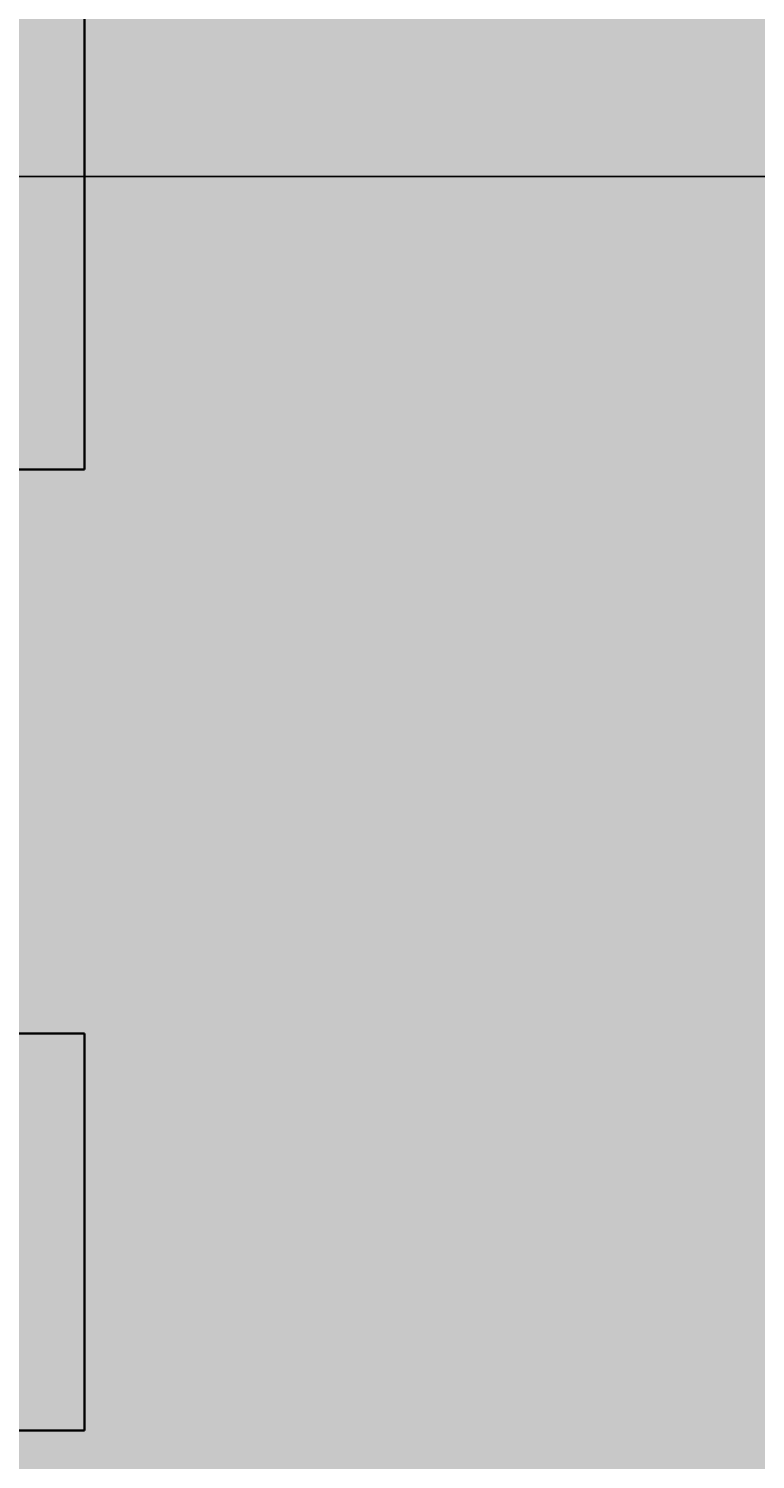
# Model space of a CAD drawing. Units: millimetres. Extents: x -229 to 16545, y -10488 to 4272.
# Tile 10 of 29: x 5862 to 7347, y -1268 to 1656. Entities that reach past the tile are written whole.
import ezdxf

# ---------------------------------------------------------------- set-up
doc = ezdxf.new("R2010")
doc.units = ezdxf.units.MM
doc.layers.add('A-ANNO-DIMS', color=2, linetype='Continuous', lineweight=18)
doc.layers.add('A-WALL', color=7, linetype='Continuous', lineweight=35)
doc.layers.add('A-FLOR-PATT', color=254, linetype='Continuous', lineweight=13, true_color=0xfeeab9)
doc.layers.add('A-WALL-PATT', color=18, linetype='Continuous', lineweight=13, true_color=0x000000)
doc.styles.get("Standard").update_dxf_attribs({"font": 'arial.ttf'})
doc.dimstyles.get("Standard").update_dxf_attribs({"dimtxt": 0.18, "dimasz": 0.18, "dimexe": 0.18, "dimexo": 0.0625, "dimgap": 0.09, "dimtad": 0, "dimtih": 1, "dimtoh": 1, "dimdec": 4, "dimzin": 0, "dimdsep": 46, "dimtxsty": 'Standard', "dimcen": 0.09, "dimadec": 0, "dimazin": 0, "dimtfac": 1, "dimtdec": 4, "dimtofl": 0, "dimtmove": 0, "dimatfit": 3, "dimfxl": 1, "dimtolj": 1, "dimtzin": 0, "dimarcsym": 0})

# ---------------------------------------------------------------- blocks, each defined once
blk = doc.blocks.new('*D85')
at = {"layer": 'A-ANNO-DIMS', "color": 0, "lineweight": -2, "transparency": 16777216}
for p, q in [((5745.9, 755.6), (5745.9, 4271.7)), ((5746.1, 4271.5), (5860.6, 4271.5)), ((5975.8, 4271.5), (5861.2, 4271.5)), ((5975.9, 755.6), (5975.9, 4271.7))]:
    blk.add_line(p, q, dxfattribs=at)
at = {"layer": 'A-ANNO-DIMS', "color": 0, "transparency": 16777216}
for points in [[(5746.1, 4271.5), (5746.1, 4271.4), (5745.9, 4271.5)], [(5975.8, 4271.5), (5975.8, 4271.4), (5975.9, 4271.5)]]:
    blk.add_solid(points, dxfattribs=at)
at = {"layer": 'Defpoints', "color": 0, "transparency": 16777216}
for p in [(5975.9, 4271.5), (5745.9, 755.5), (5975.9, 755.5)]:
    blk.add_point(p, dxfattribs=at)
at = {"layer": 'A-ANNO-DIMS', "color": 0, "transparency": 16777216, "insert": (5860.9, 4271.5), "char_height": 0.18, "attachment_point": 5}
blk.add_mtext('\\A1;230', dxfattribs=at)
blk = doc.blocks.new('*D100')
at = {"layer": 'A-ANNO-DIMS', "color": 0, "lineweight": -2, "transparency": 16777216}
for p, q in [((7294.4, 2021.7), (-228.8, 2021.7)), ((-228.7, 2021.5), (-228.7, 1688.2)), ((-228.7, 1354.6), (-228.7, 1687.9)), ((8024.8, 1354.4), (-228.8, 1354.4))]:
    blk.add_line(p, q, dxfattribs=at)
at = {"layer": 'A-ANNO-DIMS', "color": 0, "transparency": 16777216}
for points in [[(-228.7, 2021.5), (-228.6, 2021.5), (-228.7, 2021.7)], [(-228.7, 1354.6), (-228.6, 1354.6), (-228.7, 1354.4)]]:
    blk.add_solid(points, dxfattribs=at)
at = {"layer": 'Defpoints', "color": 0, "transparency": 16777216}
for p in [(7294.4, 2021.7), (-228.7, 1354.4), (8024.9, 1354.4)]:
    blk.add_point(p, dxfattribs=at)
at = {"layer": 'A-ANNO-DIMS', "color": 0, "transparency": 16777216, "insert": (-228.7, 1688.1), "char_height": 0.18, "attachment_point": 5}
blk.add_mtext('\\A1;667.3', dxfattribs=at)

msp = doc.modelspace()

# ---------------------------------------------------------------- hatches: boundary and pattern name
at = {"layer": 'A-FLOR-PATT', "transparency": 33554592}
h = msp.add_hatch(color=256, dxfattribs=at)
h.dxf.hatch_style = 1
h.paths.add_polyline_path([(7975.933, -5325.772), (7943.121, -5325.772), (7943.121, -4576.49, 0.40145271), (7225.933, -5325.772, 0.40145271), (6508.746, -4576.49), (6508.746, -5325.772), (6475.933, -5325.772), (6475.933, -5438.272), (5975.933, -5438.272), (5975.933, -7267.724), (5975.933, -7438.272), (6478.619, -7438.272), (6463.448, -7355.919), (6464.88, -7356.837), (6463.849, -7358.097), (6478.619, -7438.272), (6610.327, -7438.272), (6632.656, -7409.564), (6632.525, -7406.967), (6634.208, -7407.569), (6619.273, -7426.77), (6654.466, -7438.272), (7610.517, -7438.272), (7607.41, -7421.409), (7608.842, -7422.327), (7607.812, -7423.587), (7610.517, -7438.272), (7975.933, -7438.272)])
h.paths.add_polyline_path([(13785.933, -1208.272), (9555.933, -1208.272), (9555.933, -961.785), (9705.933, -961.785), (9705.933, -918.035), (10704.976, -918.035, 0.40145271), (9705.933, 38.215), (9555.933, 38.215), (9555.933, 2021.728), (5975.933, 2021.728), (5975.933, 755.492), (5745.933, 755.492), (5745.933, 1427.266), (2918.813, 1427.266), (2918.813, -492.942), (5013.319, -492.942), (5013.319, -978.272), (5745.933, -978.272), (5745.933, -397.513), (5975.933, -397.513), (5975.933, -1208.272), (4560.933, -1208.272), (4560.933, -1265.772), (4448.433, -1265.772), (4448.433, -1298.585), (4445.933, -1298.585), (3699.151, -1298.585, 0.40145271), (4448.433, -2015.772), (4560.933, -2015.772), (4560.933, -2384.177), (5745.933, -2384.177), (5799.402, -2384.177), (5799.402, -4518.272), (5975.933, -4518.272), (5975.933, -5208.272), (6475.933, -5208.272), (6475.933, -4575.772), (6508.746, -4575.772), (6508.746, -4576.49, -0.35647263), (7216.672, -5208.272), (7235.194, -5208.272, -0.35647263), (7943.121, -4576.49), (7943.121, -4575.772), (7975.933, -4575.772), (7975.933, -5208.272), (11176.247, -5208.272), (11159.44, -5191.465), (10520.768, -5191.465), (10520.768, -4888.936), (10571.19, -4888.936), (10571.19, -4872.129), (10772.876, -4872.129), (10772.876, -4888.936), (10789.683, -4888.936), (10789.683, -4872.129), (10991.368, -4872.129), (10991.368, -4888.936), (11041.79, -4888.936), (11041.79, -4872.129), (11058.597, -4872.129, -0.09090909), (11428.354, -4872.129), (11445.162, -4872.129), (11445.162, -4888.936), (11529.197, -4888.936), (11529.197, -5191.465), (11327.512, -5191.465), (11310.704, -5208.272), (13785.933, -5208.272)])
h.paths.add_polyline_path([(11047.216, -1630.944, -1), (11402.816, -1630.944, -1)], flags=16)
h.paths.add_polyline_path([(11148.816, -1630.944), (11225.016, -1554.744), (11301.216, -1630.944), (11225.016, -1707.144)], flags=0)
h.paths.add_polyline_path([(11199.616, -1630.944, -1), (11250.416, -1630.944, -1)], flags=0)
h.paths.add_polyline_path([(11588.751, -2096.259), (11588.751, -1543.254, -0.26666697), (12864.918, -1543.254), (12864.918, -2096.259), (12737.302, -2096.259), (12737.302, -2063.121), (11716.368, -2063.121), (11716.368, -2096.259)], flags=16)
h.paths.add_polyline_path([(12012.696, -2489.42), (12600.997, -2489.42), (12600.997, -3666.022), (12012.696, -3666.022)], flags=16)
h.paths.add_polyline_path([(12176.41, -3599.403), (12174.938, -3609.076), (12173.789, -3618.819), (12173.09, -3628.559), (12172.973, -3638.221), (12173.89, -3652.852), (12175.008, -3657.025), (12172.909, -3643.473), (12173.142, -3624.297), (12175.386, -3605.273)], flags=0)
h.paths.add_polyline_path([(8026.289, -286.944), (7737.703, -287.19), (7734.87, -269.156), (8029.092, -268.905)], flags=16)
h.paths.add_polyline_path([(7733.453, -260.139), (7710.784, -115.865), (7557.191, -115.996), (7556.999, 109.744), (7412.687, 132.166), (7412.433, 429.206), (7556.707, 451.876), (7556.568, 614.769), (7412.256, 637.19), (7412.003, 934.231), (7556.276, 956.9), (7556.084, 1182.639), (7709.677, 1182.77), (7732.099, 1327.082), (8029.14, 1327.335), (8051.808, 1183.062), (8205.401, 1183.192), (8205.594, 957.454), (8349.906, 935.031), (8350.159, 637.99), (8205.885, 615.322), (8206.024, 452.43), (8350.336, 430.006), (8350.59, 132.965), (8206.316, 110.298), (8206.509, -115.442), (8052.916, -115.573), (8030.493, -259.885)], flags=16)
h.paths.add_polyline_path([(12261.416, -3475.554), (12262.632, -3486.776), (12264.032, -3497.007), (12265.554, -3506.365), (12267.136, -3514.968), (12268.719, -3522.935), (12271.304, -3535.59), (12273.606, -3548.078), (12275.271, -3561.064), (12275.93, -3574.938), (12275.325, -3590.3), (12273.425, -3607.964), (12270.795, -3625.658), (12268.066, -3641.063), (12266.318, -3649.679), (12265.456, -3653.626), (12263.984, -3659.846), (12264.032, -3659.566), (12264.342, -3658.241), (12264.807, -3656.37), (12265.456, -3653.626), (12266.318, -3649.679), (12267.409, -3644.302), (12268.668, -3637.664), (12270.019, -3630.037), (12271.384, -3621.695), (12272.69, -3612.908), (12273.857, -3603.948), (12274.81, -3595.088), (12275.47, -3586.601), (12275.782, -3578.689), (12275.757, -3571.292), (12275.423, -3564.275), (12274.816, -3557.512), (12273.964, -3550.872), (12272.896, -3544.224), (12271.645, -3537.439), (12270.24, -3530.385), (12267.543, -3517.181), (12264.612, -3501.247), (12261.849, -3481.059)], flags=0)
h.paths.add_polyline_path([(12332.136, -3408.03), (12333.483, -3416.79), (12335.077, -3424.54), (12336.915, -3431.355), (12338.991, -3437.32), (12341.266, -3442.55), (12343.694, -3447.166), (12346.229, -3451.292), (12348.826, -3455.051), (12351.438, -3458.563), (12357.476, -3466.491), (12363.61, -3476.575), (12368.309, -3489.762), (12369.929, -3503.427), (12369.842, -3516.511), (12368.43, -3530.867), (12365.816, -3545.835), (12362.382, -3559.786), (12360.968, -3564.487), (12363.063, -3557.021), (12364.898, -3549.566), (12366.473, -3542.077), (12367.773, -3534.631), (12368.781, -3527.301), (12369.483, -3520.162), (12369.863, -3513.291), (12369.906, -3506.759), (12369.599, -3500.643), (12368.93, -3494.999), (12367.924, -3489.796), (12366.61, -3484.994), (12365.024, -3480.542), (12363.19, -3476.399), (12361.141, -3472.516), (12358.909, -3468.847), (12356.525, -3465.347), (12354.02, -3461.954), (12351.438, -3458.563), (12345.462, -3450.529), (12339.923, -3439.996), (12335.85, -3428.296), (12332.68, -3412.888)], flags=0)
h.paths.add_polyline_path([(12385.287, -3334.612), (12384.977, -3342.409), (12385.02, -3349.196), (12385.4, -3355.066), (12386.104, -3360.105), (12387.112, -3364.41), (12388.412, -3368.071), (12389.987, -3371.181), (12391.823, -3373.832), (12393.919, -3376.097), (12396.337, -3377.978), (12399.153, -3379.462), (12402.445, -3380.531), (12406.289, -3381.172), (12410.758, -3381.371), (12415.935, -3381.106), (12421.893, -3380.368), (12428.658, -3379.159), (12436.069, -3377.55), (12443.907, -3375.635), (12451.961, -3373.505), (12460.015, -3371.254), (12467.853, -3368.971), (12475.263, -3366.749), (12482.029, -3364.68), (12491.877, -3361.657), (12497.701, -3360.107), (12501.639, -3359.288), (12510.135, -3358.326), (12519.662, -3365.412), (12524.243, -3378.911), (12523.764, -3390.7), (12520.746, -3401.577), (12514.248, -3415.634), (12511.518, -3420.418), (12515.856, -3412.154), (12519.153, -3405.024), (12521.516, -3398.804), (12523.049, -3393.276), (12523.865, -3388.212), (12524.059, -3383.441), (12523.7, -3378.958), (12522.853, -3374.815), (12521.576, -3371.054), (12519.931, -3367.722), (12517.982, -3364.865), (12515.786, -3362.529), (12513.405, -3360.758), (12510.877, -3359.588), (12508.136, -3358.982), (12505.086, -3358.897), (12501.639, -3359.288), (12497.701, -3360.107), (12493.183, -3361.309), (12487.988, -3362.851), (12476.403, -3366.408), (12463.335, -3370.326), (12447.372, -3374.788), (12431.759, -3378.604), (12418.504, -3380.974), (12405.811, -3381.624), (12394.725, -3378.025), (12388.039, -3368.367), (12385.583, -3357.877), (12384.826, -3346.204), (12385.428, -3331.059), (12385.953, -3325.719)], flags=0)
h.paths.add_polyline_path([(7880.016, 1173.969), (7880.373, 1175.495), (7880.433, 1175.851), (7879.484, 1171.818)], flags=0)
h.paths.add_polyline_path([(7802.33, 874.962), (7800.771, 885.032), (7798.932, 893.941), (7796.811, 901.774), (7794.419, 908.63), (7791.798, 914.639), (7789.002, 919.945), (7786.083, 924.686), (7783.093, 929.005), (7780.087, 933.043), (7774.996, 939.717), (7768.406, 949.37), (7762.174, 963.427), (7759.342, 978.002), (7758.629, 991.888), (7759.492, 1007.928), (7761.801, 1025.496), (7765.392, 1044.035), (7766.625, 1049.048), (7764.522, 1039.543), (7762.719, 1030.232), (7761.232, 1021.168), (7760.08, 1012.405), (7759.28, 1003.994), (7758.849, 995.988), (7758.806, 988.44), (7759.167, 981.404), (7759.942, 974.914), (7761.104, 968.936), (7762.617, 963.414), (7764.448, 958.299), (7766.559, 953.535), (7768.918, 949.073), (7771.487, 944.856), (7774.232, 940.835), (7777.115, 936.938), (7782.377, 930.041), (7787.845, 922.139), (7793.348, 911.698), (7798.042, 898.247), (7801.702, 880.527)], flags=0)
h.paths.add_polyline_path([(12519.068, -3228.534), (12519.615, -3236.235), (12520.529, -3242.343), (12521.78, -3247.103), (12523.337, -3250.758), (12525.171, -3253.556), (12527.248, -3255.709), (12529.522, -3257.296), (12531.95, -3258.361), (12534.486, -3258.949), (12537.082, -3259.11), (12539.694, -3258.888), (12542.277, -3258.329), (12544.781, -3257.478), (12547.173, -3256.388), (12549.46, -3255.129), (12550.455, -3254.517), (12555.825, -3251.109), (12557.835, -3249.942), (12565.181, -3246.404), (12574.565, -3253.032), (12576.931, -3265.022), (12576.627, -3277.425), (12575.416, -3290.819), (12574.851, -3295.392), (12575.708, -3287.593), (12576.322, -3280.806), (12576.688, -3274.939), (12576.812, -3269.899), (12576.688, -3265.593), (12576.322, -3261.932), (12575.708, -3258.822), (12574.851, -3256.172), (12573.753, -3253.905), (12572.439, -3252.005), (12570.943, -3250.474), (12569.293, -3249.309), (12567.523, -3248.513), (12565.658, -3248.083), (12563.732, -3248.022), (12561.777, -3248.328), (12559.814, -3248.989), (12557.835, -3249.942), (12555.825, -3251.109), (12553.77, -3252.413), (12551.652, -3253.78), (12549.46, -3255.129), (12543.167, -3258.594), (12532.661, -3259.485), (12524.685, -3253.923), (12520.949, -3245.152), (12519.138, -3233.042)], flags=0)
h.paths.add_polyline_path([(7741.293, 790.501), (7741.641, 799.467), (7741.584, 807.269), (7741.141, 814.015), (7740.329, 819.809), (7739.165, 824.757), (7737.667, 828.966), (7735.853, 832.541), (7733.74, 835.586), (7731.348, 838.188), (7728.71, 840.348), (7725.861, 842.052), (7722.836, 843.28), (7719.671, 844.015), (7716.4, 844.237), (7713.06, 843.932), (7709.684, 843.081), (7706.304, 841.686), (7702.923, 839.834), (7699.543, 837.629), (7696.164, 835.178), (7692.784, 832.585), (7684.718, 826.315), (7675.609, 820.63), (7664.001, 817.274), (7654.105, 821.884), (7647.171, 832.02), (7644.191, 846.522), (7646.321, 860.288), (7647.49, 864.223), (7645.946, 857.865), (7645.046, 852.044), (7644.827, 846.557), (7645.243, 841.404), (7646.221, 836.642), (7647.693, 832.318), (7649.587, 828.489), (7651.832, 825.206), (7654.359, 822.523), (7657.097, 820.49), (7659.984, 819.145), (7662.993, 818.452), (7666.108, 818.357), (7669.311, 818.809), (7672.583, 819.755), (7675.908, 821.139), (7679.268, 822.913), (7682.645, 825.021), (7686.025, 827.401), (7689.404, 829.958), (7692.784, 832.585), (7700.505, 838.509), (7709.871, 843.64), (7721.436, 844.698), (7733.277, 837.617), (7739.571, 825.214), (7741.557, 811.049), (7741.669, 795.575)], flags=0)
h.paths.add_polyline_path([(8377.641, 137.216), (8359.607, 134.382), (8359.356, 428.605), (8377.395, 425.802)], flags=16)
h.paths.add_polyline_path([(7650.715, 668.465), (7650.08, 677.319), (7649.023, 684.34), (7647.579, 689.811), (7645.785, 694.012), (7643.675, 697.228), (7641.286, 699.7), (7638.669, 701.521), (7635.876, 702.744), (7632.96, 703.419), (7629.974, 703.601), (7626.971, 703.344), (7624.004, 702.697), (7621.125, 701.717), (7618.375, 700.462), (7615.749, 699.013), (7614.561, 698.279), (7608.435, 694.382), (7606.125, 693.04), (7598.981, 689.594), (7589.669, 693.773), (7585.26, 702.856), (7584.221, 713.11), (7584.49, 724.584), (7585.863, 739.937), (7586.518, 745.277), (7585.539, 736.31), (7584.841, 728.507), (7584.424, 721.761), (7584.288, 715.966), (7584.433, 711.016), (7584.86, 706.807), (7585.567, 703.231), (7586.556, 700.186), (7587.821, 697.58), (7589.332, 695.397), (7591.053, 693.637), (7592.951, 692.3), (7594.989, 691.385), (7597.132, 690.895), (7599.346, 690.826), (7601.594, 691.18), (7603.851, 691.943), (7606.125, 693.04), (7608.435, 694.382), (7610.797, 695.885), (7613.229, 697.458), (7620.475, 701.929), (7632.001, 704.44), (7643.476, 699.417), (7648.536, 687.571), (7650.63, 673.661)], flags=0)
h.paths.add_polyline_path([(7385.628, 136.37), (7385.382, 424.956), (7403.416, 427.789), (7403.667, 133.567)], flags=16)
h.paths.add_polyline_path([(12993.884, -2257.186), (12959.588, -2257.186), (12959.588, -2125.099), (13531.966, -2125.099, -0.19047621), (13531.966, -3974.321), (12959.588, -3974.321), (12959.588, -3842.233), (12993.884, -3842.233)], flags=16)
h.paths.add_polyline_path([(13413.486, -3313.884), (13413.486, -2785.535), (13562.885, -2785.535, -0.04962821), (13562.885, -3313.884)], flags=0)
h.paths.add_polyline_path([(8377.21, 642.241), (8359.176, 639.407), (8358.925, 933.629), (8376.964, 930.826)], flags=16)
h.paths.add_polyline_path([(13086.058, -1864.83), (13086.058, -1449.84), (13501.048, -1449.84), (13501.048, -1864.83)], flags=16)
h.paths.add_polyline_path([(13305.814, -1862.197), (13302.103, -1859.624), (13298.088, -1857.068), (13293.799, -1854.536), (13289.262, -1852.031), (13284.504, -1849.559), (13279.554, -1847.125), (13274.439, -1844.735), (13269.17, -1842.389), (13263.701, -1840.081), (13257.97, -1837.797), (13251.914, -1835.525), (13245.472, -1833.252), (13238.582, -1830.968), (13231.18, -1828.66), (13223.206, -1826.315), (13209.182, -1822.458), (13204.584, -1821.48), (13217.962, -1824.773), (13235.072, -1829.804), (13248.777, -1834.349), (13260.829, -1838.869), (13274.479, -1844.63), (13289.675, -1852.101), (13302.553, -1859.704)], flags=0)
h.paths.add_polyline_path([(13428.104, -1820.994), (13419.007, -1818.141), (13409.95, -1815.4), (13400.766, -1812.747), (13391.271, -1810.151), (13376.087, -1806.251), (13370.618, -1805.019), (13386.304, -1808.794), (13405.087, -1813.928), (13423.014, -1819.354)], flags=0)
h.paths.add_polyline_path([(7385.197, 641.395), (7384.951, 929.98), (7402.986, 932.814), (7403.236, 638.592)], flags=16)
h.paths.add_polyline_path([(13262.537, -1725.526), (13253.246, -1724.74), (13244.516, -1724.117), (13235.94, -1723.625), (13223.267, -1723.062), (13217.598, -1722.912), (13231.966, -1723.397), (13248.733, -1724.359), (13266.899, -1725.895), (13272.802, -1726.502)], flags=0)
h.paths.add_polyline_path([(13191.893, -1641.137), (13208.675, -1640.506), (13214.057, -1640.258), (13197.763, -1640.936)], flags=0)
h.paths.add_polyline_path([(13097.524, -1608.457), (13114.284, -1609.031), (13120.126, -1609.105), (13103.045, -1608.71)], flags=0)
h.paths.add_polyline_path([(13465.328, -1521.577), (13473.906, -1517.015), (13481.761, -1511.636), (13492.562, -1502.076), (13495.327, -1497.933), (13485.818, -1508.858), (13470.208, -1519.547)], flags=0)
h.paths.add_polyline_path([(13175.015, -1500.891), (13184.046, -1501.807), (13192.721, -1502.52), (13201.114, -1503.034), (13209.273, -1503.351), (13217.244, -1503.476), (13225.078, -1503.41), (13232.821, -1503.16), (13240.524, -1502.728), (13248.233, -1502.117), (13255.993, -1501.322), (13263.825, -1500.293), (13271.746, -1498.974), (13279.775, -1497.305), (13287.928, -1495.229), (13296.222, -1492.688), (13304.675, -1489.622), (13313.304, -1485.975), (13322.089, -1481.727), (13330.859, -1477.028), (13339.408, -1472.063), (13347.526, -1467.02), (13355.006, -1462.087), (13364.86, -1455.202), (13367.224, -1453.299), (13358.544, -1459.754), (13343.348, -1469.775), (13326.143, -1479.767), (13309.023, -1488.045), (13292.249, -1494.129), (13276.009, -1498.264), (13260.299, -1500.88), (13244.401, -1502.51), (13228.945, -1503.378), (13213.316, -1503.508), (13197.047, -1502.876), (13180.088, -1501.481)], flags=0)
h.paths.add_polyline_path([(7733.501, 1336.101), (7736.303, 1354.14), (8024.889, 1354.386), (8027.723, 1336.352)], flags=16)
at = {"layer": 'A-WALL-PATT'}
h = msp.add_hatch(color=256, dxfattribs=at)
h.dxf.hatch_style = 1
h.paths.add_polyline_path([(7294.425, 2163.983), (7294.425, 2251.728), (4412.722, 2251.728), (4412.722, 2166.741), (4412.722, 2122.457), (4412.722, 2021.728), (7294.425, 2021.728), (7294.425, 2119.698)])
h.paths.add_polyline_path([(11407.51, 2166.741), (11407.51, 2251.728), (8296.763, 2251.728), (8296.763, 2163.983), (8296.763, 2119.698), (8296.763, 2021.728), (11407.51, 2021.728), (11407.51, 2122.457)])
h.paths.add_polyline_path([(9785.933, 2021.728), (9555.933, 2021.728), (9555.933, 38.215), (9705.933, 38.215, -0.02002407), (9785.933, 35.01)])
h.paths.add_polyline_path([(14015.933, 2251.728), (12488.002, 2251.728), (12488.002, 2166.742), (12488.002, 2122.738), (12488.002, 2021.728), (13785.933, 2021.728), (13785.933, -2305.465), (13883.903, -2305.465), (13928.188, -2305.465), (14015.933, -2305.465)])
h.paths.add_polyline_path([(13785.933, -978.272), (9785.933, -978.272), (9785.933, -961.785), (9705.933, -961.785), (9555.933, -961.785), (9555.933, -1208.272), (13785.933, -1208.272)])
h.paths.add_polyline_path([(5975.933, 2021.728), (5745.933, 2021.728), (5745.933, 755.492), (5975.933, 755.492)])
h.paths.add_polyline_path([(2245.933, 2021.728), (3420.865, 2021.728), (3420.865, 2122.457), (3420.865, 2167.104), (3420.865, 2251.728), (2015.933, 2251.728), (2015.933, -3326.811), (2100.943, -3326.811), (2155.199, -3326.811), (2245.933, -3326.811)])
h.paths.add_polyline_path([(5975.933, -397.513), (5745.933, -397.513), (5745.933, -978.272), (2245.933, -978.272), (2245.933, -1208.272), (5975.933, -1208.272)])
h.paths.add_polyline_path([(12015.17, -5208.272), (7975.933, -5208.272), (7975.933, -5325.772), (7975.933, -5438.272), (7975.933, -5596.884), (8205.933, -5596.884), (8205.933, -5438.272), (12015.17, -5438.272), (12015.17, -5337.543), (12015.17, -5293.259)])
h.paths.add_polyline_path([(5975.933, -4518.272), (4567.83, -4518.272), (4567.83, -4603.259), (4567.83, -4647.543), (4567.83, -4748.272), (5745.933, -4748.272), (5745.933, -5438.272), (5975.933, -5438.272), (6475.933, -5438.272), (6475.933, -5325.772), (6475.933, -5208.272), (5975.933, -5208.272)])
h.paths.add_polyline_path([(3765.491, -4518.272), (2245.933, -4518.272), (2245.933, -4748.272), (3765.491, -4748.272), (3765.491, -4647.543), (3765.491, -4603.259)])

# ---------------------------------------------------------------- linework, layer by layer
at = {"layer": 'A-WALL'}
for p, q in [((5975.933, 755.492), (5975.933, 2021.728)), ((5745.933, 755.492), (5975.933, 755.492)), ((5745.933, -397.513), (5975.933, -397.513)), ((5975.933, -1208.272), (5975.933, -397.513)), ((2245.933, -1208.272), (5975.933, -1208.272))]:
    msp.add_line(p, q, dxfattribs=at)

# ---------------------------------------------------------------- dimensions: what is measured, and where the dimension line sits
at = {"layer": 'A-ANNO-DIMS'}
dim = msp.add_linear_dim(base=(5975.933, 4271.479), p1=(5745.933, 755.492), p2=(5975.933, 755.492), dimstyle='Standard', override={"dimdec": 0, "dimlfac": 1, "dimrnd": 0, "dimzin": 0, "dimdsep": 46, "dimlunit": 2}, dxfattribs=at)
dim.commit()
dim.dimension.update_dxf_attribs({"geometry": '*D85', "text_midpoint": (5860.933, 4271.479)})
dim = msp.add_linear_dim(base=(-228.657, 1354.386), p1=(7294.425, 2021.728), p2=(8024.889, 1354.386), angle=90, dimstyle='Standard', override={"dimdec": 1, "dimlfac": 1, "dimrnd": 0, "dimzin": 0, "dimdsep": 46, "dimlunit": 2}, dxfattribs=at)
dim.commit()
dim.dimension.update_dxf_attribs({"geometry": '*D100', "text_midpoint": (-228.657, 1688.057)})

doc.saveas('drawing.dxf')
